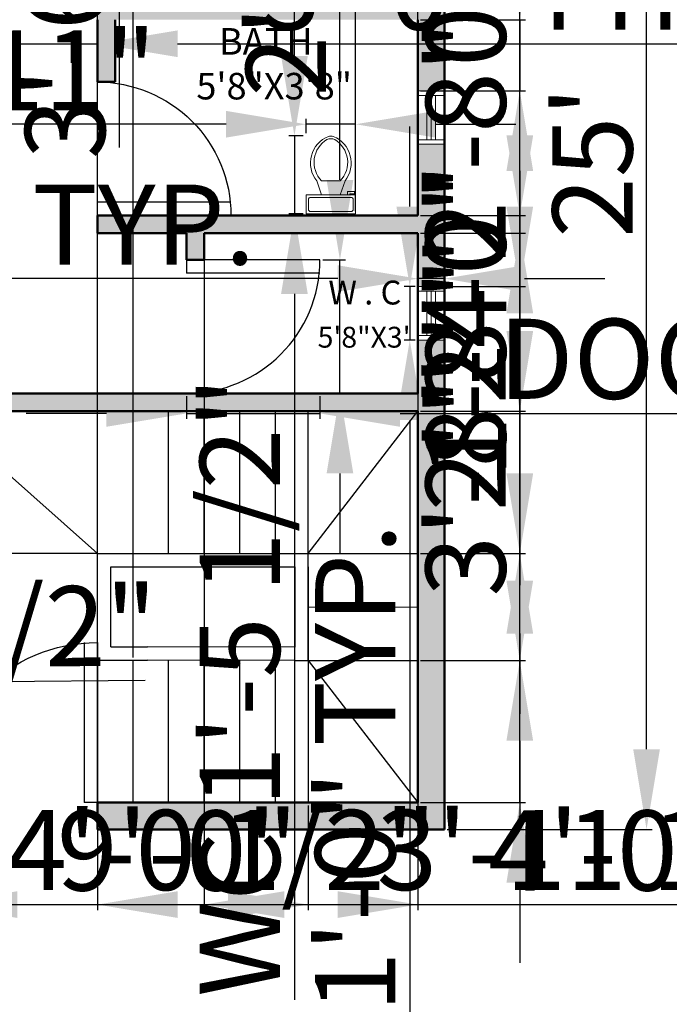
# Model space of a CAD drawing. Units: inches. Extents: x -261 to 409, y 193 to 762.
# Tile 4 of 6: x 113 to 259, y 384 to 605. Entities that reach past the tile are written whole.
import ezdxf

# ---------------------------------------------------------------- set-up
doc = ezdxf.new("R2010")
doc.units = ezdxf.units.IN
for name, color, linetype, lineweight in [('A-ANNO-DIMS', 2, 'Continuous', 18), ('A-AREA-IDEN', 7, 'Continuous', 25), ('A-DOOR', 3, 'Continuous', 25), ('A-FLOR-FIXT', 9, 'Continuous', 18), ('A-FLOR-STRS', 7, 'Continuous', 25), ('A-GLAZ', 4, 'Continuous', 18), ('A-WALL', 7, 'Continuous', 50), ('A-WALL-PATT', 8, 'Continuous', 13)]:
    doc.layers.add(name, color=color, linetype=linetype, lineweight=lineweight)
doc.styles.get("Standard").update_dxf_attribs({"font": 'arial.ttf'})
doc.dimstyles.new('ISO-25', dxfattribs={"dimtxt": 18, "dimasz": 18, "dimexe": 1.25, "dimexo": 0.625, "dimtad": 1, "dimdec": 1, "dimlunit": 3, "dimtxsty": 'Standard', "dimcen": 2.5, "dimadec": 0, "dimazin": 0, "dimtfac": 1, "dimtdec": 1, "dimtmove": 0, "dimatfit": 3, "dimfxl": 1, "dimarcsym": 0})

# ---------------------------------------------------------------- blocks, each defined once
blk = doc.blocks.new('Toilet - top')
for p, q in [((9.5, -6), (9.5, -2)), ((-8, -8.5), (-8, -8)), ((-7, -8), (-7, -9.5)), ((-4, -8), (-6, -14)), ((4, -8), (6, -14)), ((-10, -8.5), (-8, -8.5)), ((-10, -9.5), (-10, -8.5)), ((-7, -9.5), (-10, -9.5)), ((4, -14), (-4, -14))]:
    blk.add_line(p, q)
blk.add_lwpolyline([(10.5, -8), (10.5, 0), (-10.5, 0), (-10.5, -8)], close=True)
for points in [[(-9.5, -2), (-9.5, -6)], [(8.5, -1), (-8.5, -1)], [(-8.5, -7), (8.5, -7)]]:
    blk.add_lwpolyline(points)
for centre, radius, start, end in [((-8.62, -1.88), 0.884, 81.8699, 188.1301), ((8.62, -1.88), 0.884, 351.8699, 98.1301), ((-8.62, -6.12), 0.884, 171.8699, 278.1301), ((8.62, -6.12), 0.884, 261.8699, 8.1301), ((3.52, -21.58), 12.17, 141.4691, 247.9714), ((4.2, -21.82), 11.33, 136.3677, 238.9468), ((-3.52, -21.58), 12.17, 292.0284, 38.5307), ((-4.2, -21.82), 11.33, 301.053, 43.6321), ((0, -27.88), 4, 245.7318, 294.2682), ((0, -29), 4, 254.8605, 285.1395)]:
    blk.add_arc(centre, radius, start, end)
blk = doc.blocks.new('*D6')
at = {"layer": 'A-ANNO-DIMS', "color": 0, "lineweight": -2, "transparency": 16777216}
for p, q in [((208.93, 723.26), (254.96, 723.26)), ((253.71, 441.26), (253.71, 705.26)), ((208.93, 423.26), (254.96, 423.26))]:
    blk.add_line(p, q, dxfattribs=at)
at = {"layer": 'A-ANNO-DIMS', "color": 0, "transparency": 16777216}
for points in [[(250.71, 705.26), (256.71, 705.26), (253.71, 723.26)], [(250.71, 441.26), (256.71, 441.26), (253.71, 423.26)]]:
    blk.add_solid(points, dxfattribs=at)
at = {"layer": 'Defpoints', "color": 0, "transparency": 16777216}
for p in [(208.3, 723.26), (253.71, 723.26), (208.3, 423.26)]:
    blk.add_point(p, dxfattribs=at)
at = {"layer": 'A-ANNO-DIMS', "color": 0, "transparency": 16777216, "insert": (243.89, 573.26), "char_height": 18, "attachment_point": 5, "rotation": 90}
blk.add_mtext("25'", dxfattribs=at)
blk = doc.blocks.new('DOOR-SWING-36IN')
for p, q in [((0, 3), (36, 3)), ((36, 0), (36, 3)), ((0, 0), (36, 0))]:
    blk.add_line(p, q)
blk.add_arc((36, 0), 36, 90, 180)
blk = doc.blocks.new('DOOR-SWING-30IN')
for p, q in [((30, 30), (0, 30)), ((0, 30), (0, 27)), ((30, 27), (0, 27))]:
    blk.add_line(p, q)
blk.add_arc((0, 30), 30, 270, 0)
blk = doc.blocks.new('WIN-12IN')
for p, q in [((6, 12), (0, 12)), ((0, 12), (0, 0)), ((6, 0), (6, 12)), ((6, 11), (0, 11)), ((2, 1), (2, 11)), ((3, 1), (3, 11)), ((4, 1), (4, 11)), ((0, 1), (6, 1)), ((0, 0), (6, 0))]:
    blk.add_line(p, q)
blk = doc.blocks.new('*D11')
at = {"layer": 'A-ANNO-DIMS', "color": 0, "lineweight": -2, "transparency": 16777216}
for p, q in [((88.9, 659.26), (88.9, 677.26)), ((93.68, 641.26), (87.65, 641.26)), ((88.9, 641.26), (88.9, 605.26)), ((93.68, 605.26), (87.65, 605.26)), ((88.9, 587.26), (88.9, 376.77))]:
    blk.add_line(p, q, dxfattribs=at)
at = {"layer": 'A-ANNO-DIMS', "color": 0, "transparency": 16777216}
for points in [[(85.9, 659.26), (91.9, 659.26), (88.9, 641.26)], [(85.9, 587.26), (91.9, 587.26), (88.9, 605.26)]]:
    blk.add_solid(points, dxfattribs=at)
at = {"layer": 'Defpoints', "color": 0, "transparency": 16777216}
for p in [(94.3, 641.26), (88.9, 605.26), (94.3, 605.26)]:
    blk.add_point(p, dxfattribs=at)
at = {"layer": 'A-ANNO-DIMS', "color": 0, "transparency": 16777216, "insert": (78.96, 473.02), "char_height": 18, "attachment_point": 5, "rotation": 90}
blk.add_mtext('DOOR 3\'-0" TYP.', dxfattribs=at)
blk = doc.blocks.new('*D12')
at = {"layer": 'A-ANNO-DIMS', "color": 0, "lineweight": -2, "transparency": 16777216}
for p, q in [((94.3, 604.64), (94.3, 598.61)), ((130.3, 604.64), (130.3, 598.61)), ((76.3, 599.86), (58.3, 599.86)), ((94.3, 599.86), (130.3, 599.86)), ((148.3, 599.86), (277.26, 599.86))]:
    blk.add_line(p, q, dxfattribs=at)
at = {"layer": 'A-ANNO-DIMS', "color": 0, "transparency": 16777216}
for points in [[(76.3, 602.86), (76.3, 596.86), (94.3, 599.86)], [(148.3, 602.86), (148.3, 596.86), (130.3, 599.86)]]:
    blk.add_solid(points, dxfattribs=at)
at = {"layer": 'Defpoints', "color": 0, "transparency": 16777216}
for p in [(94.3, 605.26), (130.3, 605.26), (130.3, 599.86)]:
    blk.add_point(p, dxfattribs=at)
at = {"layer": 'A-ANNO-DIMS', "color": 0, "transparency": 16777216, "insert": (221.78, 609.69), "char_height": 18, "attachment_point": 5}
blk.add_mtext('3\'-0" TYP.', dxfattribs=at)
blk = doc.blocks.new('*D13')
at = {"layer": 'A-ANNO-DIMS', "color": 0, "lineweight": -2, "transparency": 16777216}
for p, q in [((150.3, 520.64), (150.3, 515.51)), ((180.3, 520.64), (180.3, 515.51)), ((132.3, 516.76), (114.3, 516.76)), ((150.3, 516.76), (180.3, 516.76)), ((198.3, 516.76), (408.8, 516.76))]:
    blk.add_line(p, q, dxfattribs=at)
at = {"layer": 'A-ANNO-DIMS', "color": 0, "transparency": 16777216}
for points in [[(132.3, 519.76), (132.3, 513.76), (150.3, 516.76)], [(198.3, 519.76), (198.3, 513.76), (180.3, 516.76)]]:
    blk.add_solid(points, dxfattribs=at)
at = {"layer": 'Defpoints', "color": 0, "transparency": 16777216}
for p in [(150.3, 521.26), (180.3, 521.26), (180.3, 516.76)]:
    blk.add_point(p, dxfattribs=at)
at = {"layer": 'A-ANNO-DIMS', "color": 0, "transparency": 16777216, "insert": (312.55, 526.7), "char_height": 18, "attachment_point": 5}
blk.add_mtext('DOOR 2\'-6" TYP.', dxfattribs=at)
blk = doc.blocks.new('*D14')
at = {"layer": 'A-ANNO-DIMS', "color": 0, "lineweight": -2, "transparency": 16777216}
for p, q in [((184.8, 569.26), (184.8, 698.54)), ((180.93, 551.26), (186.05, 551.26)), ((184.8, 521.26), (184.8, 551.26)), ((180.93, 521.26), (186.05, 521.26)), ((184.8, 503.26), (184.8, 485.26))]:
    blk.add_line(p, q, dxfattribs=at)
at = {"layer": 'A-ANNO-DIMS', "color": 0, "transparency": 16777216}
for points in [[(181.8, 569.26), (187.8, 569.26), (184.8, 551.26)], [(181.8, 503.26), (187.8, 503.26), (184.8, 521.26)]]:
    blk.add_solid(points, dxfattribs=at)
at = {"layer": 'Defpoints', "color": 0, "transparency": 16777216}
for p in [(180.3, 551.26), (184.8, 551.26), (180.3, 521.26)]:
    blk.add_point(p, dxfattribs=at)
at = {"layer": 'A-ANNO-DIMS', "color": 0, "transparency": 16777216, "insert": (174.99, 642.9), "char_height": 18, "attachment_point": 5, "rotation": 90}
blk.add_mtext('2\'-6" TYP.', dxfattribs=at)
blk = doc.blocks.new('*D17')
at = {"layer": 'A-ANNO-DIMS', "color": 0, "lineweight": -2, "transparency": 16777216}
for p, q in [((200.5, 563.26), (200.5, 581.26)), ((201.68, 545.26), (199.25, 545.26)), ((200.5, 545.26), (200.5, 533.26)), ((201.68, 533.26), (199.25, 533.26)), ((200.5, 515.26), (200.5, 268.24))]:
    blk.add_line(p, q, dxfattribs=at)
at = {"layer": 'A-ANNO-DIMS', "color": 0, "transparency": 16777216}
for points in [[(197.5, 563.26), (203.5, 563.26), (200.5, 545.26)], [(197.5, 515.26), (203.5, 515.26), (200.5, 533.26)]]:
    blk.add_solid(points, dxfattribs=at)
at = {"layer": 'Defpoints', "color": 0, "transparency": 16777216}
for p in [(202.3, 545.26), (200.5, 533.26), (202.3, 533.26)]:
    blk.add_point(p, dxfattribs=at)
at = {"layer": 'A-ANNO-DIMS', "color": 0, "transparency": 16777216, "insert": (190.56, 382.75), "char_height": 18, "attachment_point": 5, "rotation": 90}
blk.add_mtext('WINDOW 1\'-0" TYP.', dxfattribs=at)
blk = doc.blocks.new('*D18')
at = {"layer": 'A-ANNO-DIMS', "color": 0, "lineweight": -2, "transparency": 16777216}
for p, q in [((184.3, 547.06), (55.33, 547.06)), ((202.3, 545.89), (202.3, 548.31)), ((208.3, 547.06), (202.3, 547.06)), ((208.3, 545.89), (208.3, 548.31)), ((226.3, 547.06), (244.3, 547.06))]:
    blk.add_line(p, q, dxfattribs=at)
at = {"layer": 'A-ANNO-DIMS', "color": 0, "transparency": 16777216}
for points in [[(184.3, 550.06), (184.3, 544.06), (202.3, 547.06)], [(226.3, 550.06), (226.3, 544.06), (208.3, 547.06)]]:
    blk.add_solid(points, dxfattribs=at)
at = {"layer": 'Defpoints', "color": 0, "transparency": 16777216}
for p in [(202.3, 547.06), (202.3, 545.26), (208.3, 545.26)]:
    blk.add_point(p, dxfattribs=at)
at = {"layer": 'A-ANNO-DIMS', "color": 0, "transparency": 16777216, "insert": (110.82, 556.88), "char_height": 18, "attachment_point": 5}
blk.add_mtext('0\'-6" TYP.', dxfattribs=at)
blk = doc.blocks.new('*D20')
at = {"layer": 'A-ANNO-DIMS', "color": 0, "lineweight": -2, "transparency": 16777216}
for p, q in [((142.93, 685.47), (133.93, 685.47)), ((135.18, 667.47), (135.18, 661.61)), ((142.93, 643.61), (133.93, 643.61)), ((135.18, 643.61), (135.18, 576.52))]:
    blk.add_line(p, q, dxfattribs=at)
at = {"layer": 'A-ANNO-DIMS', "color": 0, "transparency": 16777216}
for points in [[(132.18, 667.47), (138.18, 667.47), (135.18, 685.47)], [(132.18, 661.61), (138.18, 661.61), (135.18, 643.61)]]:
    blk.add_solid(points, dxfattribs=at)
at = {"layer": 'Defpoints', "color": 0, "transparency": 16777216}
for p in [(143.56, 685.47), (135.18, 643.61), (143.56, 643.61)]:
    blk.add_point(p, dxfattribs=at)
at = {"layer": 'A-ANNO-DIMS', "color": 0, "transparency": 16777216, "insert": (125.36, 601.06), "char_height": 18, "attachment_point": 5, "rotation": 90}
blk.add_mtext('3\'-6"', dxfattribs=at)
blk = doc.blocks.new('*D22')
at = {"layer": 'A-ANNO-DIMS', "color": 0, "lineweight": -2, "transparency": 16777216}
for p, q in [((-11.37, 465.69), (-11.28, 454.31)), ((31.94, 466.04), (32.03, 454.66)), ((32.02, 455.91), (141.05, 456.79)), ((6.71, 455.71), (14.02, 455.77))]:
    blk.add_line(p, q, dxfattribs=at)
at = {"layer": 'A-ANNO-DIMS', "color": 0, "transparency": 16777216}
for points in [[(6.68, 458.71), (6.73, 452.71), (-11.29, 455.56)], [(14, 458.77), (14.05, 452.77), (32.02, 455.91)]]:
    blk.add_solid(points, dxfattribs=at)
at = {"layer": 'Defpoints', "color": 0, "transparency": 16777216}
for p in [(-11.38, 466.31), (31.94, 466.66), (32.02, 455.91)]:
    blk.add_point(p, dxfattribs=at)
at = {"layer": 'A-ANNO-DIMS', "color": 0, "transparency": 16777216, "insert": (95.45, 466.36), "char_height": 18, "attachment_point": 5, "rotation": 0.4625}
blk.add_mtext('3\'-7 1/2"', dxfattribs=at)
blk = doc.blocks.new('*D23')
at = {"layer": 'A-ANNO-DIMS', "color": 0, "lineweight": -2, "transparency": 16777216}
for p, q in [((174.57, 597.13), (174.57, 615.13)), ((176.57, 579.13), (173.32, 579.13)), ((174.57, 579.13), (174.57, 561.62)), ((176.57, 561.62), (173.32, 561.62)), ((174.57, 543.62), (174.57, 384.96))]:
    blk.add_line(p, q, dxfattribs=at)
at = {"layer": 'A-ANNO-DIMS', "color": 0, "transparency": 16777216}
for points in [[(171.57, 597.13), (177.57, 597.13), (174.57, 579.13)], [(171.57, 543.62), (177.57, 543.62), (174.57, 561.62)]]:
    blk.add_solid(points, dxfattribs=at)
at = {"layer": 'Defpoints', "color": 0, "transparency": 16777216}
for p in [(177.2, 579.13), (174.57, 561.62), (177.2, 561.62)]:
    blk.add_point(p, dxfattribs=at)
at = {"layer": 'A-ANNO-DIMS', "color": 0, "transparency": 16777216, "insert": (164.64, 455.29), "char_height": 18, "attachment_point": 5, "rotation": 90}
blk.add_mtext('WC 1\'-5 1/2"', dxfattribs=at)
blk = doc.blocks.new('*D24')
at = {"layer": 'A-ANNO-DIMS', "color": 0, "lineweight": -2, "transparency": 16777216}
for p, q in [((177.2, 579.75), (177.2, 583.01)), ((188.32, 579.75), (188.32, 583.01)), ((159.2, 581.76), (78.11, 581.76)), ((188.32, 581.76), (177.2, 581.76)), ((206.32, 581.76), (224.32, 581.76))]:
    blk.add_line(p, q, dxfattribs=at)
at = {"layer": 'A-ANNO-DIMS', "color": 0, "transparency": 16777216}
for points in [[(159.2, 584.76), (159.2, 578.76), (177.2, 581.76)], [(206.32, 584.76), (206.32, 578.76), (188.32, 581.76)]]:
    blk.add_solid(points, dxfattribs=at)
at = {"layer": 'Defpoints', "color": 0, "transparency": 16777216}
for p in [(177.2, 581.76), (177.2, 579.13), (188.32, 579.13)]:
    blk.add_point(p, dxfattribs=at)
at = {"layer": 'A-ANNO-DIMS', "color": 0, "transparency": 16777216, "insert": (109.65, 591.57), "char_height": 18, "attachment_point": 5}
blk.add_mtext('0\'-11"', dxfattribs=at)
blk = doc.blocks.new('*D28')
at = {"layer": 'A-ANNO-DIMS', "color": 0, "lineweight": -2, "transparency": 16777216}
for p, q in [((45.8, 422.64), (45.8, 405.1)), ((94.3, 422.64), (94.3, 405.1)), ((63.8, 406.35), (76.3, 406.35)), ((94.3, 406.35), (204.07, 406.35))]:
    blk.add_line(p, q, dxfattribs=at)
at = {"layer": 'A-ANNO-DIMS', "color": 0, "transparency": 16777216}
for points in [[(63.8, 409.35), (63.8, 403.35), (45.8, 406.35)], [(76.3, 409.35), (76.3, 403.35), (94.3, 406.35)]]:
    blk.add_solid(points, dxfattribs=at)
at = {"layer": 'Defpoints', "color": 0, "transparency": 16777216}
for p in [(45.8, 423.26), (94.3, 423.26), (94.3, 406.35)]:
    blk.add_point(p, dxfattribs=at)
at = {"layer": 'A-ANNO-DIMS', "color": 0, "transparency": 16777216, "insert": (158.19, 416.28), "char_height": 18, "attachment_point": 5}
blk.add_mtext('4\'-0 1/2"', dxfattribs=at)
blk = doc.blocks.new('*D29')
at = {"layer": 'A-ANNO-DIMS', "color": 0, "lineweight": -2, "transparency": 16777216}
for p, q in [((225.22, 479.18), (225.22, 546.58)), ((202.93, 461.18), (226.47, 461.18)), ((225.22, 429.26), (225.22, 461.18)), ((202.93, 429.26), (226.47, 429.26)), ((225.22, 411.26), (225.22, 393.26))]:
    blk.add_line(p, q, dxfattribs=at)
at = {"layer": 'A-ANNO-DIMS', "color": 0, "transparency": 16777216}
for points in [[(222.22, 479.18), (228.22, 479.18), (225.22, 461.18)], [(222.22, 411.26), (228.22, 411.26), (225.22, 429.26)]]:
    blk.add_solid(points, dxfattribs=at)
at = {"layer": 'Defpoints', "color": 0, "transparency": 16777216}
for p in [(202.3, 461.18), (225.22, 461.18), (202.3, 429.26)]:
    blk.add_point(p, dxfattribs=at)
at = {"layer": 'A-ANNO-DIMS', "color": 0, "transparency": 16777216, "insert": (215.4, 521.88), "char_height": 18, "attachment_point": 5, "rotation": 90}
blk.add_mtext('2\'-8"', dxfattribs=at)
blk = doc.blocks.new('*D32')
at = {"layer": 'A-ANNO-DIMS', "color": 0, "lineweight": -2, "transparency": 16777216}
for p, q in [((208.93, 589.26), (226.47, 589.26)), ((225.22, 571.26), (225.22, 563.26)), ((208.93, 545.26), (226.47, 545.26)), ((225.22, 545.26), (225.22, 478.18))]:
    blk.add_line(p, q, dxfattribs=at)
at = {"layer": 'A-ANNO-DIMS', "color": 0, "transparency": 16777216}
for points in [[(222.22, 571.26), (228.22, 571.26), (225.22, 589.26)], [(222.22, 563.26), (228.22, 563.26), (225.22, 545.26)]]:
    blk.add_solid(points, dxfattribs=at)
at = {"layer": 'Defpoints', "color": 0, "transparency": 16777216}
for p in [(208.3, 589.26), (208.3, 545.26), (225.22, 545.26)]:
    blk.add_point(p, dxfattribs=at)
at = {"layer": 'A-ANNO-DIMS', "color": 0, "transparency": 16777216, "insert": (215.39, 502.72), "char_height": 18, "attachment_point": 5, "rotation": 90}
blk.add_mtext('3\'-8"', dxfattribs=at)
blk = doc.blocks.new('*D33')
at = {"layer": 'A-ANNO-DIMS', "color": 0, "lineweight": -2, "transparency": 16777216}
for p, q in [((225.22, 623.26), (225.22, 641.26)), ((202.93, 605.26), (226.47, 605.26)), ((225.22, 605.26), (225.22, 589.26)), ((202.93, 589.26), (226.47, 589.26)), ((225.22, 571.26), (225.22, 505.86))]:
    blk.add_line(p, q, dxfattribs=at)
at = {"layer": 'A-ANNO-DIMS', "color": 0, "transparency": 16777216}
for points in [[(222.22, 623.26), (228.22, 623.26), (225.22, 605.26)], [(222.22, 571.26), (228.22, 571.26), (225.22, 589.26)]]:
    blk.add_solid(points, dxfattribs=at)
at = {"layer": 'Defpoints', "color": 0, "transparency": 16777216}
for p in [(202.3, 605.26), (202.3, 589.26), (225.22, 589.26)]:
    blk.add_point(p, dxfattribs=at)
at = {"layer": 'A-ANNO-DIMS', "color": 0, "transparency": 16777216, "insert": (215.55, 529.56), "char_height": 18, "attachment_point": 5, "rotation": 90}
blk.add_mtext('1\'-4"', dxfattribs=at)
blk = doc.blocks.new('*D34')
at = {"layer": 'A-ANNO-DIMS', "color": 0, "lineweight": -2, "transparency": 16777216}
for p, q in [((94.3, 428.64), (94.3, 405.1)), ((202.3, 428.64), (202.3, 405.1)), ((112.3, 406.35), (184.3, 406.35))]:
    blk.add_line(p, q, dxfattribs=at)
at = {"layer": 'A-ANNO-DIMS', "color": 0, "transparency": 16777216}
for points in [[(112.3, 409.35), (112.3, 403.35), (94.3, 406.35)], [(184.3, 409.35), (184.3, 403.35), (202.3, 406.35)]]:
    blk.add_solid(points, dxfattribs=at)
at = {"layer": 'Defpoints', "color": 0, "transparency": 16777216}
for p in [(94.3, 429.26), (202.3, 429.26), (202.3, 406.35)]:
    blk.add_point(p, dxfattribs=at)
at = {"layer": 'A-ANNO-DIMS', "color": 0, "transparency": 16777216, "insert": (148.3, 416.17), "char_height": 18, "attachment_point": 5}
blk.add_mtext('9\'-0"', dxfattribs=at)
blk = doc.blocks.new('*D37')
at = {"layer": 'A-ANNO-DIMS', "color": 0, "lineweight": -2, "transparency": 16777216}
for p, q in [((154.3, 556.64), (154.3, 405.1)), ((202.3, 556.64), (202.3, 405.1)), ((172.3, 406.35), (184.3, 406.35)), ((202.3, 406.35), (270.13, 406.35))]:
    blk.add_line(p, q, dxfattribs=at)
at = {"layer": 'A-ANNO-DIMS', "color": 0, "transparency": 16777216}
for points in [[(172.3, 409.35), (172.3, 403.35), (154.3, 406.35)], [(184.3, 409.35), (184.3, 403.35), (202.3, 406.35)]]:
    blk.add_solid(points, dxfattribs=at)
at = {"layer": 'Defpoints', "color": 0, "transparency": 16777216}
for p in [(154.3, 557.26), (202.3, 557.26), (202.3, 406.35)]:
    blk.add_point(p, dxfattribs=at)
at = {"layer": 'A-ANNO-DIMS', "color": 0, "transparency": 16777216, "insert": (245.21, 416.17), "char_height": 18, "attachment_point": 5}
blk.add_mtext('4\'-0"', dxfattribs=at)
blk = doc.blocks.new('*D38')
at = {"layer": 'A-ANNO-DIMS', "color": 0, "lineweight": -2, "transparency": 16777216}
for p, q in [((225.22, 579.26), (225.22, 646.36)), ((202.93, 561.26), (226.47, 561.26)), ((225.22, 557.26), (225.22, 561.26)), ((202.93, 557.26), (226.47, 557.26)), ((225.22, 539.26), (225.22, 521.26))]:
    blk.add_line(p, q, dxfattribs=at)
at = {"layer": 'A-ANNO-DIMS', "color": 0, "transparency": 16777216}
for points in [[(222.22, 579.26), (228.22, 579.26), (225.22, 561.26)], [(222.22, 539.26), (228.22, 539.26), (225.22, 557.26)]]:
    blk.add_solid(points, dxfattribs=at)
at = {"layer": 'Defpoints', "color": 0, "transparency": 16777216}
for p in [(202.3, 561.26), (225.22, 561.26), (202.3, 557.26)]:
    blk.add_point(p, dxfattribs=at)
at = {"layer": 'A-ANNO-DIMS', "color": 0, "transparency": 16777216, "insert": (215.4, 621.81), "char_height": 18, "attachment_point": 5, "rotation": 90}
blk.add_mtext('0\'-4"', dxfattribs=at)
blk = doc.blocks.new('*D39')
at = {"layer": 'A-ANNO-DIMS', "color": 0, "lineweight": -2, "transparency": 16777216}
for p, q in [((225.22, 503.26), (225.22, 570.67)), ((202.93, 485.26), (226.47, 485.26)), ((225.22, 461.18), (225.22, 485.26)), ((202.93, 461.18), (226.47, 461.18)), ((225.22, 443.18), (225.22, 425.18))]:
    blk.add_line(p, q, dxfattribs=at)
at = {"layer": 'A-ANNO-DIMS', "color": 0, "transparency": 16777216}
for points in [[(222.22, 503.26), (228.22, 503.26), (225.22, 485.26)], [(222.22, 443.18), (228.22, 443.18), (225.22, 461.18)]]:
    blk.add_solid(points, dxfattribs=at)
at = {"layer": 'Defpoints', "color": 0, "transparency": 16777216}
for p in [(202.3, 485.26), (225.22, 485.26), (202.3, 461.18)]:
    blk.add_point(p, dxfattribs=at)
at = {"layer": 'A-ANNO-DIMS', "color": 0, "transparency": 16777216, "insert": (215.4, 545.97), "char_height": 18, "attachment_point": 5, "rotation": 90}
blk.add_mtext('2\'-0"', dxfattribs=at)
blk = doc.blocks.new('*D40')
at = {"layer": 'A-ANNO-DIMS', "color": 0, "lineweight": -2, "transparency": 16777216}
for p, q in [((225.22, 535.26), (225.22, 602.67)), ((202.93, 517.26), (226.47, 517.26)), ((225.22, 485.26), (225.22, 517.26)), ((202.93, 485.26), (226.47, 485.26)), ((225.22, 467.26), (225.22, 449.26))]:
    blk.add_line(p, q, dxfattribs=at)
at = {"layer": 'A-ANNO-DIMS', "color": 0, "transparency": 16777216}
for points in [[(222.22, 535.26), (228.22, 535.26), (225.22, 517.26)], [(222.22, 467.26), (228.22, 467.26), (225.22, 485.26)]]:
    blk.add_solid(points, dxfattribs=at)
at = {"layer": 'Defpoints', "color": 0, "transparency": 16777216}
for p in [(202.3, 517.26), (225.22, 517.26), (202.3, 485.26)]:
    blk.add_point(p, dxfattribs=at)
at = {"layer": 'A-ANNO-DIMS', "color": 0, "transparency": 16777216, "insert": (215.4, 577.97), "char_height": 18, "attachment_point": 5, "rotation": 90}
blk.add_mtext('2\'-8"', dxfattribs=at)
blk = doc.blocks.new('*D41')
at = {"layer": 'A-ANNO-DIMS', "color": 0, "lineweight": -2, "transparency": 16777216}
for p, q in [((130.3, 428.64), (130.3, 405.1)), ((177.66, 428.64), (177.66, 405.1)), ((148.3, 406.35), (159.66, 406.35)), ((177.66, 406.35), (300.67, 406.35))]:
    blk.add_line(p, q, dxfattribs=at)
at = {"layer": 'A-ANNO-DIMS', "color": 0, "transparency": 16777216}
for points in [[(148.3, 409.35), (148.3, 403.35), (130.3, 406.35)], [(159.66, 409.35), (159.66, 403.35), (177.66, 406.35)]]:
    blk.add_solid(points, dxfattribs=at)
at = {"layer": 'Defpoints', "color": 0, "transparency": 16777216}
for p in [(130.3, 429.26), (177.66, 429.26), (177.66, 406.35)]:
    blk.add_point(p, dxfattribs=at)
at = {"layer": 'A-ANNO-DIMS', "color": 0, "transparency": 16777216, "insert": (248.17, 416.29), "char_height": 18, "attachment_point": 5}
blk.add_mtext('3\'-11 1/2"', dxfattribs=at)
blk = doc.blocks.new('*D42')
at = {"layer": 'A-ANNO-DIMS', "color": 0, "lineweight": -2, "transparency": 16777216}
for p, q in [((112.3, 740.18), (94.3, 740.18)), ((130.3, 461.89), (130.3, 741.43)), ((130.3, 740.18), (138.3, 740.18)), ((138.3, 461.89), (138.3, 741.43)), ((156.3, 740.18), (223.4, 740.18))]:
    blk.add_line(p, q, dxfattribs=at)
at = {"layer": 'A-ANNO-DIMS', "color": 0, "transparency": 16777216}
for points in [[(112.3, 743.18), (112.3, 737.18), (130.3, 740.18)], [(156.3, 743.18), (156.3, 737.18), (138.3, 740.18)]]:
    blk.add_solid(points, dxfattribs=at)
at = {"layer": 'Defpoints', "color": 0, "transparency": 16777216}
for p in [(138.3, 740.18), (130.3, 461.26), (138.3, 461.26)]:
    blk.add_point(p, dxfattribs=at)
at = {"layer": 'A-ANNO-DIMS', "color": 0, "transparency": 16777216, "insert": (198.85, 749.99), "char_height": 18, "attachment_point": 5}
blk.add_mtext('0\'-8"', dxfattribs=at)
blk = doc.blocks.new('*D44')
at = {"layer": 'A-ANNO-DIMS', "color": 0, "lineweight": -2, "transparency": 16777216}
for p, q in [((170.32, 740.18), (152.32, 740.18)), ((188.32, 562.25), (188.32, 741.43)), ((188.32, 740.18), (202.3, 740.18)), ((202.3, 561.89), (202.3, 741.43)), ((220.3, 740.18), (285.71, 740.18))]:
    blk.add_line(p, q, dxfattribs=at)
at = {"layer": 'A-ANNO-DIMS', "color": 0, "transparency": 16777216}
for points in [[(170.32, 743.18), (170.32, 737.18), (188.32, 740.18)], [(220.3, 743.18), (220.3, 737.18), (202.3, 740.18)]]:
    blk.add_solid(points, dxfattribs=at)
at = {"layer": 'Defpoints', "color": 0, "transparency": 16777216}
for p in [(202.3, 740.18), (188.32, 561.62), (202.3, 561.26)]:
    blk.add_point(p, dxfattribs=at)
at = {"layer": 'A-ANNO-DIMS', "color": 0, "transparency": 16777216, "insert": (262.01, 749.84), "char_height": 18, "attachment_point": 5}
blk.add_mtext('1\'-2"', dxfattribs=at)

msp = doc.modelspace()

# ---------------------------------------------------------------- hatches: boundary and pattern name
at = {"layer": 'A-WALL-PATT'}
h = msp.add_hatch(color=256, dxfattribs=at)
h.dxf.hatch_style = 1
h.paths.add_polyline_path([(-25.7, 675.26), (-16.7, 675.26), (-16.7, 681.26), (-31.7, 681.26), (-31.7, 423.26), (-14.2, 423.26), (-14.2, 429.26), (-25.7, 429.26), (-25.7, 569.26), (52.3, 569.26), (88.3, 569.26), (94.3, 569.26), (94.3, 573.26), (52.3, 573.26), (-25.7, 573.26), (-25.7, 575.26)])
h.paths.add_polyline_path([(94.3, 429.26), (58.3, 429.26), (45.8, 429.26), (45.8, 423.26), (94.3, 423.26)])
h.paths.add_polyline_path([(208.3, 533.26), (202.3, 533.26), (202.3, 521.26), (150.3, 521.26), (94.3, 521.26), (94.3, 531.26), (88.3, 531.26), (88.3, 465.26), (94.3, 465.26), (94.3, 517.26), (150.3, 517.26), (202.3, 517.26), (202.3, 429.26), (130.3, 429.26), (130.3, 423.26), (208.3, 423.26)])
h.paths.add_polyline_path([(208.3, 577.26), (202.3, 577.26), (202.3, 561.26), (130.3, 561.26), (130.3, 557.26), (150.3, 557.26), (150.3, 551.26), (154.3, 551.26), (154.3, 557.26), (202.3, 557.26), (202.3, 545.26), (208.3, 545.26)])
h.paths.add_polyline_path([(208.3, 633.26), (202.3, 633.26), (202.3, 609.26), (130.3, 609.26), (130.3, 605.26), (130.3, 591.26), (134.3, 591.26), (134.3, 605.26), (202.3, 605.26), (202.3, 589.26), (208.3, 589.26)])
h.paths.add_polyline_path([(208.3, 723.26), (88.3, 723.26), (88.3, 605.26), (94.3, 605.26), (94.3, 641.26), (94.3, 717.26), (202.3, 717.26), (202.3, 693.26), (208.3, 693.26)])
h.paths.add_polyline_path([(52.3, 681.26), (43.3, 681.26), (43.3, 675.26), (52.3, 675.26), (52.3, 677.26)], flags=17)

# ---------------------------------------------------------------- linework, layer by layer
at = {"layer": 'A-FLOR-STRS'}
for p, q in [((130.3, 485.26), (94.3, 517.26)), ((130.3, 429.26), (130.3, 517.26)), ((138.3, 485.26), (138.3, 517.26)), ((146.3, 485.26), (146.3, 517.26)), ((154.3, 485.26), (154.3, 517.26)), ((162.3, 485.26), (162.3, 517.26)), ((170.3, 485.26), (170.3, 517.26)), ((177.66, 461.18), (177.66, 517.26)), ((177.67, 485.26), (202.3, 517.26)), ((130.3, 485.26), (94.3, 485.26)), ((130.3, 485.26), (141.56, 485.26)), ((141.56, 485.26), (174.67, 485.26)), ((174.67, 485.26), (177.67, 485.26)), ((177.66, 485.26), (202.3, 485.26)), ((177.67, 482.26), (177.67, 485.26)), ((133.3, 482.26), (141.56, 482.26)), ((133.3, 464.26), (133.3, 482.26)), ((141.56, 482.26), (174.67, 482.26)), ((174.67, 482.26), (174.66, 464.18)), ((177.67, 482.26), (177.66, 464.17)), ((177.66, 473.22), (202.3, 473.26)), ((133.3, 464.26), (141.56, 464.26)), ((174.66, 464.18), (141.55, 464.26)), ((177.66, 464.17), (177.66, 461.18)), ((130.3, 461.26), (141.56, 461.26)), ((138.3, 429.26), (138.3, 461.26)), ((174.65, 461.18), (141.55, 461.26)), ((146.3, 429.26), (146.3, 461.25)), ((154.3, 429.26), (154.3, 461.23)), ((162.3, 429.26), (162.3, 461.21)), ((170.3, 429.26), (170.3, 461.19)), ((174.65, 461.18), (177.66, 461.18)), ((177.66, 461.18), (177.66, 429.26)), ((177.66, 461.18), (202.3, 461.18)), ((177.66, 461.18), (202.3, 429.26))]:
    msp.add_line(p, q, dxfattribs=at)
at = {"layer": 'A-WALL'}
for p, q in [((208.3, 423.26), (208.3, 723.26)), ((130.3, 591.26), (130.3, 605.26)), ((134.3, 591.26), (134.3, 605.26)), ((202.3, 561.26), (202.3, 605.26)), ((134.3, 591.26), (130.3, 591.26)), ((202.3, 561.26), (130.3, 561.26)), ((130.3, 557.26), (130.3, 561.26)), ((150.3, 557.26), (130.3, 557.26)), ((150.3, 551.26), (150.3, 557.26)), ((202.3, 557.26), (154.3, 557.26)), ((154.3, 551.26), (154.3, 557.26)), ((202.3, 521.26), (202.3, 557.26)), ((154.3, 551.26), (150.3, 551.26)), ((150.3, 521.26), (94.3, 521.26)), ((202.3, 521.26), (150.3, 521.26)), ((150.3, 517.26), (94.3, 517.26)), ((202.3, 517.26), (150.3, 517.26)), ((202.3, 429.26), (202.3, 517.26)), ((130.3, 429.26), (130.3, 423.26)), ((130.3, 429.26), (202.3, 429.26)), ((130.3, 423.26), (208.3, 423.26))]:
    msp.add_line(p, q, dxfattribs=at)

# ---------------------------------------------------------------- block references
at = {"layer": 'A-DOOR', "extrusion": (0, 0, -1), "zscale": -1}
for name, p, rotation in [('DOOR-SWING-30IN', (-130.3, 591.26), 180), ('DOOR-SWING-36IN', (-130.3, 465.26), 269.9999999999998)]:
    msp.add_blockref(name, p, dxfattribs=dict(at, rotation=rotation))
at = {"layer": 'A-DOOR'}
msp.add_blockref('DOOR-SWING-30IN', (150.3, 521.26), dxfattribs=at)
at = {"layer": 'A-FLOR-FIXT', "xscale": 0.5297904838490288, "yscale": 0.5297904838490288, "zscale": 0.5297904838490288, "rotation": 180}
msp.add_blockref('Toilet - top', (182.76, 561.62), dxfattribs=at)
at = {"layer": 'A-GLAZ', "rotation": 180}
for p in [(208.3, 589.26), (208.3, 545.26)]:
    msp.add_blockref('WIN-12IN', p, dxfattribs=at)

# ---------------------------------------------------------------- texts
at = {"layer": 'A-AREA-IDEN', "attachment_point": 1}
for s, width, gutter_width, insert, char_height in [('BATH', 143.7583, 29.83, (157.6, 603.37), 5.965), ('5\'8"X3\'8"', 143.7583, 29.83, (152.53, 593.31), 5.965), ('W . C', 129.3158, 26.83, (182.19, 546.61), 5.366), ('5\'8"X3\'', 112.9106, 23.43, (179.79, 536.23), 4.685)]:
    msp.add_mtext_dynamic_manual_height_columns(s, width=width, gutter_width=gutter_width, heights=[0], dxfattribs=dict(at, insert=insert, char_height=char_height))

# ---------------------------------------------------------------- dimensions: what is measured, and where the dimension line sits
at = {"layer": 'A-ANNO-DIMS'}
for base, p1, p2, picture, middle in [((138.3, 740.18), (130.3, 461.26), (138.3, 461.26), '*D42', (198.85, 749.99)), ((202.3, 740.18), (188.32, 561.62), (202.3, 561.26), '*D44', (262.01, 749.84)), ((202.3, 406.35), (154.3, 557.26), (202.3, 557.26), '*D37', (245.21, 416.17)), ((94.3, 406.35), (45.8, 423.26), (94.3, 423.26), '*D28', (158.19, 416.28)), ((177.66, 406.35), (130.3, 429.26), (177.66, 429.26), '*D41', (248.17, 416.29)), ((202.3, 406.35), (94.3, 429.26), (202.3, 429.26), '*D34', (148.3, 416.17))]:
    dim = msp.add_linear_dim(base=base, p1=p1, p2=p2, dimstyle='ISO-25', override={"dimdec": 1, "dimlfac": 1, "dimrnd": 0, "dimzin": 1, "dimdsep": 46, "dimlunit": 4, "dimfrac": 2}, dxfattribs=at)
    dim.commit()
    dim.dimension.update_dxf_attribs({"geometry": picture, "text_midpoint": middle})
for base, p1, p2, angle, override, picture, middle in [((253.71, 723.26), (208.3, 423.26), (208.3, 723.26), 90, {"dimclrd": 0, "dimclre": 0, "dimclrt": 0}, '*D6', (243.89, 573.26)), ((135.18, 643.61), (143.56, 685.47), (143.56, 643.61), 270, {"dimdec": 1, "dimlfac": 1, "dimrnd": 0, "dimzin": 1, "dimdsep": 46, "dimlunit": 4, "dimfrac": 2}, '*D20', (125.36, 601.06)), ((225.22, 561.26), (202.3, 557.26), (202.3, 561.26), 90, {"dimdec": 1, "dimlfac": 1, "dimrnd": 0, "dimzin": 1, "dimdsep": 46, "dimlunit": 4, "dimfrac": 2}, '*D38', (215.4, 621.81)), ((225.22, 589.26), (202.3, 605.26), (202.3, 589.26), 90, {"dimdec": 1, "dimlfac": 1, "dimrnd": 0, "dimzin": 1, "dimdsep": 46, "dimlunit": 4, "dimfrac": 2}, '*D33', (215.55, 529.56)), ((225.22, 517.26), (202.3, 485.26), (202.3, 517.26), 90, {"dimdec": 1, "dimlfac": 1, "dimrnd": 0, "dimzin": 1, "dimdsep": 46, "dimlunit": 4, "dimfrac": 2}, '*D40', (215.4, 577.97)), ((177.2, 581.76), (188.32, 579.13), (177.2, 579.13), 180, {"dimdec": 1, "dimlfac": 1, "dimrnd": 0, "dimzin": 1, "dimdsep": 46, "dimlunit": 4, "dimfrac": 2}, '*D24', (109.65, 591.57)), ((225.22, 545.26), (208.3, 589.26), (208.3, 545.26), 90, {"dimdec": 1, "dimlfac": 1, "dimrnd": 0, "dimzin": 1, "dimdsep": 46, "dimlunit": 4, "dimfrac": 2}, '*D32', (215.39, 502.72)), ((225.22, 485.26), (202.3, 461.18), (202.3, 485.26), 90, {"dimdec": 1, "dimlfac": 1, "dimrnd": 0, "dimzin": 1, "dimdsep": 46, "dimlunit": 4, "dimfrac": 2}, '*D39', (215.4, 545.97)), ((225.22, 461.18), (202.3, 429.26), (202.3, 461.18), 90, {"dimdec": 1, "dimlfac": 1, "dimrnd": 0, "dimzin": 1, "dimdsep": 46, "dimlunit": 4, "dimfrac": 2}, '*D29', (215.4, 521.88)), ((32.02, 455.91), (-11.38, 466.31), (31.94, 466.66), 0.4625, {"dimdec": 1, "dimlfac": 1, "dimrnd": 0, "dimzin": 1, "dimdsep": 46, "dimlunit": 4, "dimfrac": 2}, '*D22', (95.45, 466.36))]:
    dim = msp.add_linear_dim(base=base, p1=p1, p2=p2, angle=angle, dimstyle='ISO-25', override=override, dxfattribs=at)
    dim.commit()
    dim.dimension.update_dxf_attribs({"geometry": picture, "text_midpoint": middle})
for base, p1, p2, angle, text, picture, middle in [((184.8, 551.26), (180.3, 521.26), (180.3, 551.26), 90, '<> TYP.', '*D14', (174.99, 642.9)), ((88.9, 605.26), (94.3, 641.26), (94.3, 605.26), 270, 'DOOR <> TYP.', '*D11', (78.96, 473.02)), ((174.57, 561.62), (177.2, 579.13), (177.2, 561.62), 270, 'WC <>', '*D23', (164.64, 455.29)), ((202.3, 547.06), (208.3, 545.26), (202.3, 545.26), 180, '<> TYP.', '*D18', (110.82, 556.88)), ((200.5, 533.26), (202.3, 545.26), (202.3, 533.26), 270, 'WINDOW <> TYP.', '*D17', (190.56, 382.75))]:
    dim = msp.add_linear_dim(base=base, p1=p1, p2=p2, angle=angle, text=text, dimstyle='ISO-25', override={"dimdec": 1, "dimlfac": 1, "dimrnd": 0, "dimzin": 1, "dimdsep": 46, "dimlunit": 4, "dimfrac": 2}, dxfattribs=at)
    dim.commit()
    dim.dimension.update_dxf_attribs({"geometry": picture, "text_midpoint": middle})
for base, p1, p2, text, picture, middle in [((130.3, 599.86), (94.3, 605.26), (130.3, 605.26), '<> TYP.', '*D12', (221.78, 609.69)), ((180.3, 516.76), (150.3, 521.26), (180.3, 521.26), 'DOOR <> TYP.', '*D13', (312.55, 526.7))]:
    dim = msp.add_linear_dim(base=base, p1=p1, p2=p2, text=text, dimstyle='ISO-25', override={"dimdec": 1, "dimlfac": 1, "dimrnd": 0, "dimzin": 1, "dimdsep": 46, "dimlunit": 4, "dimfrac": 2}, dxfattribs=at)
    dim.commit()
    dim.dimension.update_dxf_attribs({"geometry": picture, "text_midpoint": middle})

doc.saveas('drawing.dxf')
